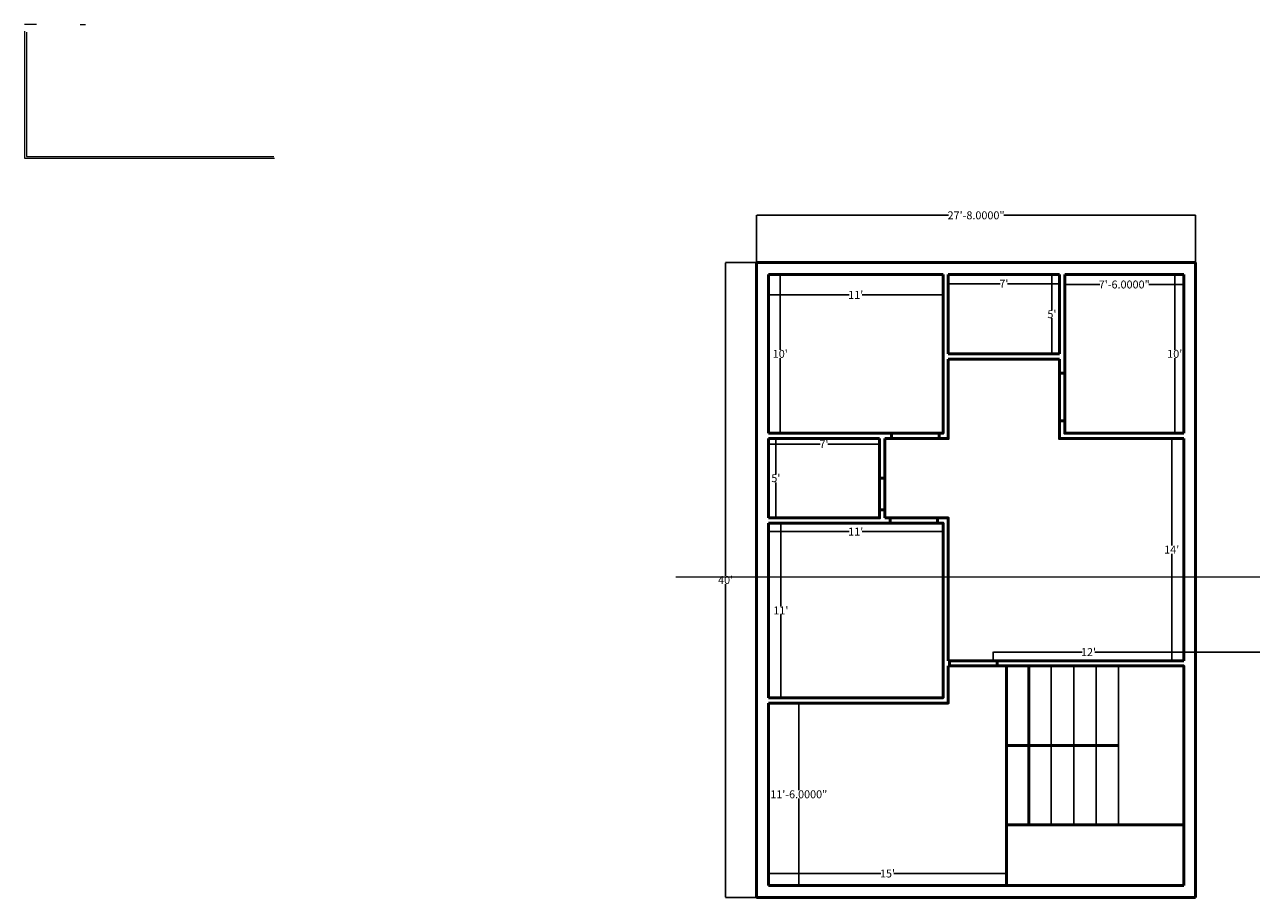
# Model space of a CAD drawing. Units: feet. Extents: x 993 to 3080, y -271 to 22562.
# Tile 2 of 4: x 993 to 1920, y 557 to 1217. Entities that reach past the tile are written whole.
import ezdxf

# ---------------------------------------------------------------- set-up
doc = ezdxf.new("R2010")
doc.units = ezdxf.units.FT
for name, color, linetype, lineweight in [('A-ANNO-DIMS', 2, 'Continuous', 18), ('A-ANNO-NPLT', 9, 'Continuous', 13), ('A-ANNO-SYMB', 4, 'Continuous', 18), ('A-FLOR-STRS', 3, 'Continuous', 25), ('A-WALL', 7, 'Continuous', 50)]:
    doc.layers.add(name, color=color, linetype=linetype, lineweight=lineweight)
doc.styles.get("Standard").update_dxf_attribs({"font": 'arial.ttf'})
doc.dimstyles.get("Standard").update_dxf_attribs({"dimtxt": 6, "dimasz": 0.18, "dimexe": 0.18, "dimexo": 0.0625, "dimgap": 0.09, "dimtad": 0, "dimtih": 1, "dimtoh": 1, "dimdec": 4, "dimzin": 0, "dimdsep": 46, "dimlunit": 3, "dimtxsty": 'Standard', "dimcen": 0.09, "dimadec": 0, "dimazin": 0, "dimtfac": 1, "dimtdec": 4, "dimtofl": 0, "dimtmove": 0, "dimatfit": 3, "dimfxl": 1, "dimtolj": 1, "dimtzin": 0, "dimarcsym": 0})

# ---------------------------------------------------------------- blocks, each defined once
blk = doc.blocks.new('*D1')
at = {"layer": 'A-ANNO-DIMS', "color": 0, "lineweight": -2, "transparency": 16777216}
for p, q in [((1545.92, 1037.12), (1545.92, 1072.98)), ((1546.1, 1072.8), (1690.98, 1072.8)), ((1877.74, 1072.8), (1732.85, 1072.8)), ((1877.92, 1037.12), (1877.92, 1072.98))]:
    blk.add_line(p, q, dxfattribs=at)
at = {"layer": 'A-ANNO-DIMS', "color": 0, "transparency": 16777216}
for points in [[(1546.1, 1072.83), (1546.1, 1072.77), (1545.92, 1072.8)], [(1877.74, 1072.83), (1877.74, 1072.77), (1877.92, 1072.8)]]:
    blk.add_solid(points, dxfattribs=at)
at = {"layer": 'Defpoints', "color": 0, "transparency": 16777216}
for p in [(1877.92, 1072.8), (1545.92, 1037.06), (1877.92, 1037.06)]:
    blk.add_point(p, dxfattribs=at)
at = {"layer": 'A-ANNO-DIMS', "color": 0, "transparency": 16777216, "insert": (1711.92, 1072.8), "char_height": 6, "attachment_point": 5}
blk.add_mtext('\\A1;27\'-8.0000"', dxfattribs=at)
blk = doc.blocks.new('*D2')
at = {"layer": 'A-ANNO-DIMS', "color": 0, "lineweight": -2, "transparency": 16777216}
for p, q in [((1545.85, 1037.06), (1522.38, 1037.06)), ((1522.56, 1036.88), (1522.56, 800.21)), ((1522.56, 557.24), (1522.56, 793.91)), ((1545.85, 557.06), (1522.38, 557.06))]:
    blk.add_line(p, q, dxfattribs=at)
at = {"layer": 'A-ANNO-DIMS', "color": 0, "transparency": 16777216}
for points in [[(1522.53, 1036.88), (1522.59, 1036.88), (1522.56, 1037.06)], [(1522.53, 557.24), (1522.59, 557.24), (1522.56, 557.06)]]:
    blk.add_solid(points, dxfattribs=at)
at = {"layer": 'Defpoints', "color": 0, "transparency": 16777216}
for p in [(1545.92, 1037.06), (1522.56, 557.06), (1545.92, 557.06)]:
    blk.add_point(p, dxfattribs=at)
at = {"layer": 'A-ANNO-DIMS', "color": 0, "transparency": 16777216, "insert": (1522.56, 797.06), "char_height": 6, "attachment_point": 5}
blk.add_mtext("\\A1;40'", dxfattribs=at)
blk = doc.blocks.new('*D3')
at = {"layer": 'A-ANNO-DIMS', "color": 0, "lineweight": -2, "transparency": 16777216}
for p, q in [((1554.92, 1028), (1554.92, 1012.47)), ((1686.92, 1028), (1686.92, 1012.47)), ((1555.1, 1012.65), (1616.02, 1012.65)), ((1686.74, 1012.65), (1625.81, 1012.65))]:
    blk.add_line(p, q, dxfattribs=at)
at = {"layer": 'A-ANNO-DIMS', "color": 0, "transparency": 16777216}
for points in [[(1555.1, 1012.68), (1555.1, 1012.62), (1554.92, 1012.65)], [(1686.74, 1012.68), (1686.74, 1012.62), (1686.92, 1012.65)]]:
    blk.add_solid(points, dxfattribs=at)
at = {"layer": 'Defpoints', "color": 0, "transparency": 16777216}
for p in [(1554.92, 1028.06), (1686.92, 1028.06), (1686.92, 1012.65)]:
    blk.add_point(p, dxfattribs=at)
at = {"layer": 'A-ANNO-DIMS', "color": 0, "transparency": 16777216, "insert": (1620.92, 1012.65), "char_height": 6, "attachment_point": 5}
blk.add_mtext("\\A1;11'", dxfattribs=at)
blk = doc.blocks.new('*D4')
at = {"layer": 'A-ANNO-DIMS', "color": 0, "lineweight": -2, "transparency": 16777216}
for p, q in [((1554.98, 1028.06), (1564.08, 1028.06)), ((1563.9, 1027.88), (1563.9, 971.21)), ((1563.9, 908.24), (1563.9, 964.91)), ((1554.98, 908.06), (1564.08, 908.06))]:
    blk.add_line(p, q, dxfattribs=at)
at = {"layer": 'A-ANNO-DIMS', "color": 0, "transparency": 16777216}
for points in [[(1563.87, 1027.88), (1563.93, 1027.88), (1563.9, 1028.06)], [(1563.87, 908.24), (1563.93, 908.24), (1563.9, 908.06)]]:
    blk.add_solid(points, dxfattribs=at)
at = {"layer": 'Defpoints', "color": 0, "transparency": 16777216}
for p in [(1554.92, 1028.06), (1554.92, 908.06), (1563.9, 908.06)]:
    blk.add_point(p, dxfattribs=at)
at = {"layer": 'A-ANNO-DIMS', "color": 0, "transparency": 16777216, "insert": (1563.9, 968.06), "char_height": 6, "attachment_point": 5}
blk.add_mtext("\\A1;10'", dxfattribs=at)
blk = doc.blocks.new('*D5')
at = {"layer": 'A-ANNO-DIMS', "color": 0, "lineweight": -2, "transparency": 16777216}
for p, q in [((1690.92, 1028), (1690.92, 1020.88)), ((1691.1, 1021.06), (1730.09, 1021.06)), ((1774.74, 1021.06), (1735.74, 1021.06)), ((1774.92, 1028), (1774.92, 1020.88))]:
    blk.add_line(p, q, dxfattribs=at)
at = {"layer": 'A-ANNO-DIMS', "color": 0, "transparency": 16777216}
for points in [[(1691.1, 1021.09), (1691.1, 1021.03), (1690.92, 1021.06)], [(1774.74, 1021.09), (1774.74, 1021.03), (1774.92, 1021.06)]]:
    blk.add_solid(points, dxfattribs=at)
at = {"layer": 'Defpoints', "color": 0, "transparency": 16777216}
for p in [(1690.92, 1028.06), (1774.92, 1028.06), (1774.92, 1021.06)]:
    blk.add_point(p, dxfattribs=at)
at = {"layer": 'A-ANNO-DIMS', "color": 0, "transparency": 16777216, "insert": (1732.92, 1021.06), "char_height": 6, "attachment_point": 5}
blk.add_mtext("\\A1;7'", dxfattribs=at)
blk = doc.blocks.new('*D6')
at = {"layer": 'A-ANNO-DIMS', "color": 0, "lineweight": -2, "transparency": 16777216}
for p, q in [((1774.85, 1028.06), (1769.08, 1028.06)), ((1769.26, 1027.88), (1769.26, 1001.2)), ((1769.26, 968.24), (1769.26, 994.92)), ((1774.85, 968.06), (1769.08, 968.06))]:
    blk.add_line(p, q, dxfattribs=at)
at = {"layer": 'A-ANNO-DIMS', "color": 0, "transparency": 16777216}
for points in [[(1769.23, 1027.88), (1769.29, 1027.88), (1769.26, 1028.06)], [(1769.23, 968.24), (1769.29, 968.24), (1769.26, 968.06)]]:
    blk.add_solid(points, dxfattribs=at)
at = {"layer": 'Defpoints', "color": 0, "transparency": 16777216}
for p in [(1769.26, 1028.06), (1774.92, 1028.06), (1774.92, 968.06)]:
    blk.add_point(p, dxfattribs=at)
at = {"layer": 'A-ANNO-DIMS', "color": 0, "transparency": 16777216, "insert": (1769.26, 998.06), "char_height": 6, "attachment_point": 5}
blk.add_mtext("\\A1;5'", dxfattribs=at)
blk = doc.blocks.new('*D7')
at = {"layer": 'A-ANNO-DIMS', "color": 0, "lineweight": -2, "transparency": 16777216}
for p, q in [((1778.92, 1028), (1778.92, 1020.32)), ((1779.1, 1020.5), (1805.39, 1020.5)), ((1868.74, 1020.5), (1842.44, 1020.5)), ((1868.92, 1028), (1868.92, 1020.32))]:
    blk.add_line(p, q, dxfattribs=at)
at = {"layer": 'A-ANNO-DIMS', "color": 0, "transparency": 16777216}
for points in [[(1779.1, 1020.53), (1779.1, 1020.47), (1778.92, 1020.5)], [(1868.74, 1020.53), (1868.74, 1020.47), (1868.92, 1020.5)]]:
    blk.add_solid(points, dxfattribs=at)
at = {"layer": 'Defpoints', "color": 0, "transparency": 16777216}
for p in [(1778.92, 1028.06), (1778.92, 1020.5), (1868.92, 1028.06)]:
    blk.add_point(p, dxfattribs=at)
at = {"layer": 'A-ANNO-DIMS', "color": 0, "transparency": 16777216, "insert": (1823.92, 1020.5), "char_height": 6, "attachment_point": 5}
blk.add_mtext('\\A1;7\'-6.0000"', dxfattribs=at)
blk = doc.blocks.new('*D8')
at = {"layer": 'A-ANNO-DIMS', "color": 0, "lineweight": -2, "transparency": 16777216}
for p, q in [((1868.85, 1028.06), (1861.9, 1028.06)), ((1862.08, 1027.88), (1862.08, 971.21)), ((1862.08, 908.24), (1862.08, 964.91)), ((1868.85, 908.06), (1861.9, 908.06))]:
    blk.add_line(p, q, dxfattribs=at)
at = {"layer": 'A-ANNO-DIMS', "color": 0, "transparency": 16777216}
for points in [[(1862.05, 1027.88), (1862.11, 1027.88), (1862.08, 1028.06)], [(1862.05, 908.24), (1862.11, 908.24), (1862.08, 908.06)]]:
    blk.add_solid(points, dxfattribs=at)
at = {"layer": 'Defpoints', "color": 0, "transparency": 16777216}
for p in [(1868.92, 1028.06), (1862.08, 908.06), (1868.92, 908.06)]:
    blk.add_point(p, dxfattribs=at)
at = {"layer": 'A-ANNO-DIMS', "color": 0, "transparency": 16777216, "insert": (1862.08, 968.06), "char_height": 6, "attachment_point": 5}
blk.add_mtext("\\A1;10'", dxfattribs=at)
blk = doc.blocks.new('*D9')
at = {"layer": 'A-ANNO-DIMS', "color": 0, "lineweight": -2, "transparency": 16777216}
for p, q in [((1554.92, 904), (1554.92, 899.62)), ((1555.1, 899.8), (1594.09, 899.8)), ((1638.74, 899.8), (1599.74, 899.8)), ((1638.92, 904), (1638.92, 899.62))]:
    blk.add_line(p, q, dxfattribs=at)
at = {"layer": 'A-ANNO-DIMS', "color": 0, "transparency": 16777216}
for points in [[(1555.1, 899.83), (1555.1, 899.77), (1554.92, 899.8)], [(1638.74, 899.83), (1638.74, 899.77), (1638.92, 899.8)]]:
    blk.add_solid(points, dxfattribs=at)
at = {"layer": 'Defpoints', "color": 0, "transparency": 16777216}
for p in [(1554.92, 904.06), (1554.92, 899.8), (1638.92, 904.06)]:
    blk.add_point(p, dxfattribs=at)
at = {"layer": 'A-ANNO-DIMS', "color": 0, "transparency": 16777216, "insert": (1596.92, 899.8), "char_height": 6, "attachment_point": 5}
blk.add_mtext("\\A1;7'", dxfattribs=at)
blk = doc.blocks.new('*D10')
at = {"layer": 'A-ANNO-DIMS', "color": 0, "lineweight": -2, "transparency": 16777216}
for p, q in [((1554.98, 904.06), (1560.73, 904.06)), ((1560.55, 903.88), (1560.55, 877.2)), ((1560.55, 844.24), (1560.55, 870.92)), ((1554.98, 844.06), (1560.73, 844.06))]:
    blk.add_line(p, q, dxfattribs=at)
at = {"layer": 'A-ANNO-DIMS', "color": 0, "transparency": 16777216}
for points in [[(1560.52, 903.88), (1560.58, 903.88), (1560.55, 904.06)], [(1560.52, 844.24), (1560.58, 844.24), (1560.55, 844.06)]]:
    blk.add_solid(points, dxfattribs=at)
at = {"layer": 'Defpoints', "color": 0, "transparency": 16777216}
for p in [(1554.92, 904.06), (1554.92, 844.06), (1560.55, 844.06)]:
    blk.add_point(p, dxfattribs=at)
at = {"layer": 'A-ANNO-DIMS', "color": 0, "transparency": 16777216, "insert": (1560.55, 874.06), "char_height": 6, "attachment_point": 5}
blk.add_mtext("\\A1;5'", dxfattribs=at)
blk = doc.blocks.new('*D11')
at = {"layer": 'A-ANNO-DIMS', "color": 0, "lineweight": -2, "transparency": 16777216}
for p, q in [((1554.98, 840.06), (1564.54, 840.06)), ((1564.36, 839.88), (1564.36, 777.16)), ((1564.36, 708.24), (1564.36, 770.96)), ((1554.98, 708.06), (1564.54, 708.06))]:
    blk.add_line(p, q, dxfattribs=at)
at = {"layer": 'A-ANNO-DIMS', "color": 0, "transparency": 16777216}
for points in [[(1564.33, 839.88), (1564.39, 839.88), (1564.36, 840.06)], [(1564.33, 708.24), (1564.39, 708.24), (1564.36, 708.06)]]:
    blk.add_solid(points, dxfattribs=at)
at = {"layer": 'Defpoints', "color": 0, "transparency": 16777216}
for p in [(1554.92, 840.06), (1554.92, 708.06), (1564.36, 708.06)]:
    blk.add_point(p, dxfattribs=at)
at = {"layer": 'A-ANNO-DIMS', "color": 0, "transparency": 16777216, "insert": (1564.36, 774.06), "char_height": 6, "attachment_point": 5}
blk.add_mtext("\\A1;11'", dxfattribs=at)
blk = doc.blocks.new('*D12')
at = {"layer": 'A-ANNO-DIMS', "color": 0, "lineweight": -2, "transparency": 16777216}
for p, q in [((1554.92, 840), (1554.92, 833.46)), ((1686.92, 840), (1686.92, 833.46)), ((1555.1, 833.64), (1616.02, 833.64)), ((1686.74, 833.64), (1625.81, 833.64))]:
    blk.add_line(p, q, dxfattribs=at)
at = {"layer": 'A-ANNO-DIMS', "color": 0, "transparency": 16777216}
for points in [[(1555.1, 833.67), (1555.1, 833.61), (1554.92, 833.64)], [(1686.74, 833.67), (1686.74, 833.61), (1686.92, 833.64)]]:
    blk.add_solid(points, dxfattribs=at)
at = {"layer": 'Defpoints', "color": 0, "transparency": 16777216}
for p in [(1554.92, 840.06), (1686.92, 840.06), (1686.92, 833.64)]:
    blk.add_point(p, dxfattribs=at)
at = {"layer": 'A-ANNO-DIMS', "color": 0, "transparency": 16777216, "insert": (1620.92, 833.64), "char_height": 6, "attachment_point": 5}
blk.add_mtext("\\A1;11'", dxfattribs=at)
blk = doc.blocks.new('*D13')
at = {"layer": 'A-ANNO-DIMS', "color": 0, "lineweight": -2, "transparency": 16777216}
for p, q in [((1868.85, 904.06), (1859.63, 904.06)), ((1859.81, 903.88), (1859.81, 823.16)), ((1859.81, 736.24), (1859.81, 816.96)), ((1868.85, 736.06), (1859.63, 736.06))]:
    blk.add_line(p, q, dxfattribs=at)
at = {"layer": 'A-ANNO-DIMS', "color": 0, "transparency": 16777216}
for points in [[(1859.78, 903.88), (1859.84, 903.88), (1859.81, 904.06)], [(1859.78, 736.24), (1859.84, 736.24), (1859.81, 736.06)]]:
    blk.add_solid(points, dxfattribs=at)
at = {"layer": 'Defpoints', "color": 0, "transparency": 16777216}
for p in [(1868.92, 904.06), (1859.81, 736.06), (1868.92, 736.06)]:
    blk.add_point(p, dxfattribs=at)
at = {"layer": 'A-ANNO-DIMS', "color": 0, "transparency": 16777216, "insert": (1859.81, 820.06), "char_height": 6, "attachment_point": 5}
blk.add_mtext("\\A1;14'", dxfattribs=at)
blk = doc.blocks.new('*D14')
at = {"layer": 'A-ANNO-DIMS', "color": 0, "lineweight": -2, "transparency": 16777216}
for p, q in [((1724.92, 736.12), (1724.92, 742.78)), ((1725.1, 742.6), (1792.02, 742.6)), ((1868.74, 742.6), (1801.81, 742.6)), ((1868.92, 736.12), (1868.92, 742.78))]:
    blk.add_line(p, q, dxfattribs=at)
at = {"layer": 'A-ANNO-DIMS', "color": 0, "transparency": 16777216}
for points in [[(1725.1, 742.63), (1725.1, 742.57), (1724.92, 742.6)], [(1868.74, 742.63), (1868.74, 742.57), (1868.92, 742.6)]]:
    blk.add_solid(points, dxfattribs=at)
at = {"layer": 'Defpoints', "color": 0, "transparency": 16777216}
for p in [(1724.92, 742.6), (1724.92, 736.06), (1868.92, 736.06)]:
    blk.add_point(p, dxfattribs=at)
at = {"layer": 'A-ANNO-DIMS', "color": 0, "transparency": 16777216, "insert": (1796.92, 742.6), "char_height": 6, "attachment_point": 5}
blk.add_mtext("\\A1;12'", dxfattribs=at)
blk = doc.blocks.new('*D15')
at = {"layer": 'A-ANNO-DIMS', "color": 0, "lineweight": -2, "transparency": 16777216}
for p, q in [((1554.98, 704.06), (1578.06, 704.06)), ((1577.88, 703.88), (1577.88, 638.21)), ((1577.88, 566.24), (1577.88, 631.91)), ((1554.98, 566.06), (1578.06, 566.06))]:
    blk.add_line(p, q, dxfattribs=at)
at = {"layer": 'A-ANNO-DIMS', "color": 0, "transparency": 16777216}
for points in [[(1577.85, 703.88), (1577.91, 703.88), (1577.88, 704.06)], [(1577.85, 566.24), (1577.91, 566.24), (1577.88, 566.06)]]:
    blk.add_solid(points, dxfattribs=at)
at = {"layer": 'Defpoints', "color": 0, "transparency": 16777216}
for p in [(1554.92, 704.06), (1554.92, 566.06), (1577.88, 566.06)]:
    blk.add_point(p, dxfattribs=at)
at = {"layer": 'A-ANNO-DIMS', "color": 0, "transparency": 16777216, "insert": (1577.88, 635.06), "char_height": 6, "attachment_point": 5}
blk.add_mtext('\\A1;11\'-6.0000"', dxfattribs=at)
blk = doc.blocks.new('*D16')
at = {"layer": 'A-ANNO-DIMS', "color": 0, "lineweight": -2, "transparency": 16777216}
for p, q in [((1554.92, 566.12), (1554.92, 575.34)), ((1555.1, 575.16), (1640.02, 575.16)), ((1734.74, 575.16), (1649.81, 575.16)), ((1734.92, 566.12), (1734.92, 575.34))]:
    blk.add_line(p, q, dxfattribs=at)
at = {"layer": 'A-ANNO-DIMS', "color": 0, "transparency": 16777216}
for points in [[(1555.1, 575.19), (1555.1, 575.13), (1554.92, 575.16)], [(1734.74, 575.19), (1734.74, 575.13), (1734.92, 575.16)]]:
    blk.add_solid(points, dxfattribs=at)
at = {"layer": 'Defpoints', "color": 0, "transparency": 16777216}
for p in [(1734.92, 575.16), (1554.92, 566.06), (1734.92, 566.06)]:
    blk.add_point(p, dxfattribs=at)
at = {"layer": 'A-ANNO-DIMS', "color": 0, "transparency": 16777216, "insert": (1644.92, 575.16), "char_height": 6, "attachment_point": 5}
blk.add_mtext("\\A1;15'", dxfattribs=at)
blk = doc.blocks.new('*D19')
at = {"layer": 'A-ANNO-DIMS', "color": 0, "lineweight": -2, "transparency": 16777216}
for p, q in [((1554.92, 1028), (1554.92, 1012.47)), ((1686.92, 1028), (1686.92, 1012.47)), ((1555.1, 1012.65), (1616.02, 1012.65)), ((1686.74, 1012.65), (1625.81, 1012.65))]:
    blk.add_line(p, q, dxfattribs=at)
at = {"layer": 'A-ANNO-DIMS', "color": 0, "transparency": 16777216}
for points in [[(1555.1, 1012.68), (1555.1, 1012.62), (1554.92, 1012.65)], [(1686.74, 1012.68), (1686.74, 1012.62), (1686.92, 1012.65)]]:
    blk.add_solid(points, dxfattribs=at)
at = {"layer": 'Defpoints', "color": 0, "transparency": 16777216}
for p in [(1554.92, 1028.06), (1686.92, 1028.06), (1686.92, 1012.65)]:
    blk.add_point(p, dxfattribs=at)
at = {"layer": 'A-ANNO-DIMS', "color": 0, "transparency": 16777216, "insert": (1620.92, 1012.65), "char_height": 6, "attachment_point": 5}
blk.add_mtext("\\A1;11'", dxfattribs=at)
blk = doc.blocks.new('*D20')
at = {"layer": 'A-ANNO-DIMS', "color": 0, "lineweight": -2, "transparency": 16777216}
for p, q in [((1554.98, 1028.06), (1564.08, 1028.06)), ((1563.9, 1027.88), (1563.9, 971.21)), ((1563.9, 908.24), (1563.9, 964.91)), ((1554.98, 908.06), (1564.08, 908.06))]:
    blk.add_line(p, q, dxfattribs=at)
at = {"layer": 'A-ANNO-DIMS', "color": 0, "transparency": 16777216}
for points in [[(1563.87, 1027.88), (1563.93, 1027.88), (1563.9, 1028.06)], [(1563.87, 908.24), (1563.93, 908.24), (1563.9, 908.06)]]:
    blk.add_solid(points, dxfattribs=at)
at = {"layer": 'Defpoints', "color": 0, "transparency": 16777216}
for p in [(1554.92, 1028.06), (1554.92, 908.06), (1563.9, 908.06)]:
    blk.add_point(p, dxfattribs=at)
at = {"layer": 'A-ANNO-DIMS', "color": 0, "transparency": 16777216, "insert": (1563.9, 968.06), "char_height": 6, "attachment_point": 5}
blk.add_mtext("\\A1;10'", dxfattribs=at)
blk = doc.blocks.new('*D21')
at = {"layer": 'A-ANNO-DIMS', "color": 0, "lineweight": -2, "transparency": 16777216}
for p, q in [((1690.92, 1028), (1690.92, 1020.88)), ((1691.1, 1021.06), (1730.09, 1021.06)), ((1774.74, 1021.06), (1735.74, 1021.06)), ((1774.92, 1028), (1774.92, 1020.88))]:
    blk.add_line(p, q, dxfattribs=at)
at = {"layer": 'A-ANNO-DIMS', "color": 0, "transparency": 16777216}
for points in [[(1691.1, 1021.09), (1691.1, 1021.03), (1690.92, 1021.06)], [(1774.74, 1021.09), (1774.74, 1021.03), (1774.92, 1021.06)]]:
    blk.add_solid(points, dxfattribs=at)
at = {"layer": 'Defpoints', "color": 0, "transparency": 16777216}
for p in [(1690.92, 1028.06), (1774.92, 1028.06), (1774.92, 1021.06)]:
    blk.add_point(p, dxfattribs=at)
at = {"layer": 'A-ANNO-DIMS', "color": 0, "transparency": 16777216, "insert": (1732.92, 1021.06), "char_height": 6, "attachment_point": 5}
blk.add_mtext("\\A1;7'", dxfattribs=at)
blk = doc.blocks.new('*D22')
at = {"layer": 'A-ANNO-DIMS', "color": 0, "lineweight": -2, "transparency": 16777216}
for p, q in [((1774.85, 1028.06), (1769.08, 1028.06)), ((1769.26, 1027.88), (1769.26, 1001.2)), ((1769.26, 968.24), (1769.26, 994.92)), ((1774.85, 968.06), (1769.08, 968.06))]:
    blk.add_line(p, q, dxfattribs=at)
at = {"layer": 'A-ANNO-DIMS', "color": 0, "transparency": 16777216}
for points in [[(1769.23, 1027.88), (1769.29, 1027.88), (1769.26, 1028.06)], [(1769.23, 968.24), (1769.29, 968.24), (1769.26, 968.06)]]:
    blk.add_solid(points, dxfattribs=at)
at = {"layer": 'Defpoints', "color": 0, "transparency": 16777216}
for p in [(1769.26, 1028.06), (1774.92, 1028.06), (1774.92, 968.06)]:
    blk.add_point(p, dxfattribs=at)
at = {"layer": 'A-ANNO-DIMS', "color": 0, "transparency": 16777216, "insert": (1769.26, 998.06), "char_height": 6, "attachment_point": 5}
blk.add_mtext("\\A1;5'", dxfattribs=at)
blk = doc.blocks.new('*D23')
at = {"layer": 'A-ANNO-DIMS', "color": 0, "lineweight": -2, "transparency": 16777216}
for p, q in [((1778.92, 1028), (1778.92, 1020.32)), ((1779.1, 1020.5), (1805.39, 1020.5)), ((1868.74, 1020.5), (1842.44, 1020.5)), ((1868.92, 1028), (1868.92, 1020.32))]:
    blk.add_line(p, q, dxfattribs=at)
at = {"layer": 'A-ANNO-DIMS', "color": 0, "transparency": 16777216}
for points in [[(1779.1, 1020.53), (1779.1, 1020.47), (1778.92, 1020.5)], [(1868.74, 1020.53), (1868.74, 1020.47), (1868.92, 1020.5)]]:
    blk.add_solid(points, dxfattribs=at)
at = {"layer": 'Defpoints', "color": 0, "transparency": 16777216}
for p in [(1778.92, 1028.06), (1778.92, 1020.5), (1868.92, 1028.06)]:
    blk.add_point(p, dxfattribs=at)
at = {"layer": 'A-ANNO-DIMS', "color": 0, "transparency": 16777216, "insert": (1823.92, 1020.5), "char_height": 6, "attachment_point": 5}
blk.add_mtext('\\A1;7\'-6.0000"', dxfattribs=at)
blk = doc.blocks.new('*D24')
at = {"layer": 'A-ANNO-DIMS', "color": 0, "lineweight": -2, "transparency": 16777216}
for p, q in [((1868.85, 1028.06), (1861.9, 1028.06)), ((1862.08, 1027.88), (1862.08, 971.21)), ((1862.08, 908.24), (1862.08, 964.91)), ((1868.85, 908.06), (1861.9, 908.06))]:
    blk.add_line(p, q, dxfattribs=at)
at = {"layer": 'A-ANNO-DIMS', "color": 0, "transparency": 16777216}
for points in [[(1862.05, 1027.88), (1862.11, 1027.88), (1862.08, 1028.06)], [(1862.05, 908.24), (1862.11, 908.24), (1862.08, 908.06)]]:
    blk.add_solid(points, dxfattribs=at)
at = {"layer": 'Defpoints', "color": 0, "transparency": 16777216}
for p in [(1868.92, 1028.06), (1862.08, 908.06), (1868.92, 908.06)]:
    blk.add_point(p, dxfattribs=at)
at = {"layer": 'A-ANNO-DIMS', "color": 0, "transparency": 16777216, "insert": (1862.08, 968.06), "char_height": 6, "attachment_point": 5}
blk.add_mtext("\\A1;10'", dxfattribs=at)
blk = doc.blocks.new('*D25')
at = {"layer": 'A-ANNO-DIMS', "color": 0, "lineweight": -2, "transparency": 16777216}
for p, q in [((1554.92, 904), (1554.92, 899.62)), ((1555.1, 899.8), (1594.09, 899.8)), ((1638.74, 899.8), (1599.74, 899.8)), ((1638.92, 904), (1638.92, 899.62))]:
    blk.add_line(p, q, dxfattribs=at)
at = {"layer": 'A-ANNO-DIMS', "color": 0, "transparency": 16777216}
for points in [[(1555.1, 899.83), (1555.1, 899.77), (1554.92, 899.8)], [(1638.74, 899.83), (1638.74, 899.77), (1638.92, 899.8)]]:
    blk.add_solid(points, dxfattribs=at)
at = {"layer": 'Defpoints', "color": 0, "transparency": 16777216}
for p in [(1554.92, 904.06), (1554.92, 899.8), (1638.92, 904.06)]:
    blk.add_point(p, dxfattribs=at)
at = {"layer": 'A-ANNO-DIMS', "color": 0, "transparency": 16777216, "insert": (1596.92, 899.8), "char_height": 6, "attachment_point": 5}
blk.add_mtext("\\A1;7'", dxfattribs=at)
blk = doc.blocks.new('*D26')
at = {"layer": 'A-ANNO-DIMS', "color": 0, "lineweight": -2, "transparency": 16777216}
for p, q in [((1554.98, 904.06), (1560.73, 904.06)), ((1560.55, 903.88), (1560.55, 877.2)), ((1560.55, 844.24), (1560.55, 870.92)), ((1554.98, 844.06), (1560.73, 844.06))]:
    blk.add_line(p, q, dxfattribs=at)
at = {"layer": 'A-ANNO-DIMS', "color": 0, "transparency": 16777216}
for points in [[(1560.52, 903.88), (1560.58, 903.88), (1560.55, 904.06)], [(1560.52, 844.24), (1560.58, 844.24), (1560.55, 844.06)]]:
    blk.add_solid(points, dxfattribs=at)
at = {"layer": 'Defpoints', "color": 0, "transparency": 16777216}
for p in [(1554.92, 904.06), (1554.92, 844.06), (1560.55, 844.06)]:
    blk.add_point(p, dxfattribs=at)
at = {"layer": 'A-ANNO-DIMS', "color": 0, "transparency": 16777216, "insert": (1560.55, 874.06), "char_height": 6, "attachment_point": 5}
blk.add_mtext("\\A1;5'", dxfattribs=at)
blk = doc.blocks.new('*D27')
at = {"layer": 'A-ANNO-DIMS', "color": 0, "lineweight": -2, "transparency": 16777216}
for p, q in [((1554.98, 840.06), (1564.54, 840.06)), ((1564.36, 839.88), (1564.36, 777.16)), ((1564.36, 708.24), (1564.36, 770.96)), ((1554.98, 708.06), (1564.54, 708.06))]:
    blk.add_line(p, q, dxfattribs=at)
at = {"layer": 'A-ANNO-DIMS', "color": 0, "transparency": 16777216}
for points in [[(1564.33, 839.88), (1564.39, 839.88), (1564.36, 840.06)], [(1564.33, 708.24), (1564.39, 708.24), (1564.36, 708.06)]]:
    blk.add_solid(points, dxfattribs=at)
at = {"layer": 'Defpoints', "color": 0, "transparency": 16777216}
for p in [(1554.92, 840.06), (1554.92, 708.06), (1564.36, 708.06)]:
    blk.add_point(p, dxfattribs=at)
at = {"layer": 'A-ANNO-DIMS', "color": 0, "transparency": 16777216, "insert": (1564.36, 774.06), "char_height": 6, "attachment_point": 5}
blk.add_mtext("\\A1;11'", dxfattribs=at)
blk = doc.blocks.new('*D28')
at = {"layer": 'A-ANNO-DIMS', "color": 0, "lineweight": -2, "transparency": 16777216}
for p, q in [((1554.92, 840), (1554.92, 833.46)), ((1686.92, 840), (1686.92, 833.46)), ((1555.1, 833.64), (1616.02, 833.64)), ((1686.74, 833.64), (1625.81, 833.64))]:
    blk.add_line(p, q, dxfattribs=at)
at = {"layer": 'A-ANNO-DIMS', "color": 0, "transparency": 16777216}
for points in [[(1555.1, 833.67), (1555.1, 833.61), (1554.92, 833.64)], [(1686.74, 833.67), (1686.74, 833.61), (1686.92, 833.64)]]:
    blk.add_solid(points, dxfattribs=at)
at = {"layer": 'Defpoints', "color": 0, "transparency": 16777216}
for p in [(1554.92, 840.06), (1686.92, 840.06), (1686.92, 833.64)]:
    blk.add_point(p, dxfattribs=at)
at = {"layer": 'A-ANNO-DIMS', "color": 0, "transparency": 16777216, "insert": (1620.92, 833.64), "char_height": 6, "attachment_point": 5}
blk.add_mtext("\\A1;11'", dxfattribs=at)
blk = doc.blocks.new('*D29')
at = {"layer": 'A-ANNO-DIMS', "color": 0, "lineweight": -2, "transparency": 16777216}
for p, q in [((1868.85, 904.06), (1859.63, 904.06)), ((1859.81, 903.88), (1859.81, 823.16)), ((1859.81, 736.24), (1859.81, 816.96)), ((1868.85, 736.06), (1859.63, 736.06))]:
    blk.add_line(p, q, dxfattribs=at)
at = {"layer": 'A-ANNO-DIMS', "color": 0, "transparency": 16777216}
for points in [[(1859.78, 903.88), (1859.84, 903.88), (1859.81, 904.06)], [(1859.78, 736.24), (1859.84, 736.24), (1859.81, 736.06)]]:
    blk.add_solid(points, dxfattribs=at)
at = {"layer": 'Defpoints', "color": 0, "transparency": 16777216}
for p in [(1868.92, 904.06), (1859.81, 736.06), (1868.92, 736.06)]:
    blk.add_point(p, dxfattribs=at)
at = {"layer": 'A-ANNO-DIMS', "color": 0, "transparency": 16777216, "insert": (1859.81, 820.06), "char_height": 6, "attachment_point": 5}
blk.add_mtext("\\A1;14'", dxfattribs=at)
blk = doc.blocks.new('*D30')
at = {"layer": 'A-ANNO-DIMS', "color": 0, "lineweight": -2, "transparency": 16777216}
for p, q in [((1868.92, 736.12), (1868.92, 742.78)), ((1869.1, 742.6), (1999, 742.6)), ((2170.78, 742.6), (2040.87, 742.6)), ((2170.96, 736.12), (2170.96, 742.78))]:
    blk.add_line(p, q, dxfattribs=at)
at = {"layer": 'A-ANNO-DIMS', "color": 0, "transparency": 16777216}
for points in [[(1869.1, 742.63), (1869.1, 742.57), (1868.92, 742.6)], [(2170.78, 742.63), (2170.78, 742.57), (2170.96, 742.6)]]:
    blk.add_solid(points, dxfattribs=at)
at = {"layer": 'Defpoints', "color": 0, "transparency": 16777216}
for p in [(2170.96, 742.6), (1868.92, 736.06), (2170.96, 736.06)]:
    blk.add_point(p, dxfattribs=at)
at = {"layer": 'A-ANNO-DIMS', "color": 0, "transparency": 16777216, "insert": (2019.94, 742.6), "char_height": 6, "attachment_point": 5}
blk.add_mtext('\\A1;25\'-2.0427"', dxfattribs=at)
blk = doc.blocks.new('*D31')
at = {"layer": 'A-ANNO-DIMS', "color": 0, "lineweight": -2, "transparency": 16777216}
for p, q in [((1554.98, 704.06), (1578.06, 704.06)), ((1577.88, 703.88), (1577.88, 638.21)), ((1577.88, 566.24), (1577.88, 631.91)), ((1554.98, 566.06), (1578.06, 566.06))]:
    blk.add_line(p, q, dxfattribs=at)
at = {"layer": 'A-ANNO-DIMS', "color": 0, "transparency": 16777216}
for points in [[(1577.85, 703.88), (1577.91, 703.88), (1577.88, 704.06)], [(1577.85, 566.24), (1577.91, 566.24), (1577.88, 566.06)]]:
    blk.add_solid(points, dxfattribs=at)
at = {"layer": 'Defpoints', "color": 0, "transparency": 16777216}
for p in [(1554.92, 704.06), (1554.92, 566.06), (1577.88, 566.06)]:
    blk.add_point(p, dxfattribs=at)
at = {"layer": 'A-ANNO-DIMS', "color": 0, "transparency": 16777216, "insert": (1577.88, 635.06), "char_height": 6, "attachment_point": 5}
blk.add_mtext('\\A1;11\'-6.0000"', dxfattribs=at)
blk = doc.blocks.new('*D32')
at = {"layer": 'A-ANNO-DIMS', "color": 0, "lineweight": -2, "transparency": 16777216}
for p, q in [((1554.92, 566.12), (1554.92, 575.34)), ((1555.1, 575.16), (1640.02, 575.16)), ((1734.74, 575.16), (1649.81, 575.16)), ((1734.92, 566.12), (1734.92, 575.34))]:
    blk.add_line(p, q, dxfattribs=at)
at = {"layer": 'A-ANNO-DIMS', "color": 0, "transparency": 16777216}
for points in [[(1555.1, 575.19), (1555.1, 575.13), (1554.92, 575.16)], [(1734.74, 575.19), (1734.74, 575.13), (1734.92, 575.16)]]:
    blk.add_solid(points, dxfattribs=at)
at = {"layer": 'Defpoints', "color": 0, "transparency": 16777216}
for p in [(1734.92, 575.16), (1554.92, 566.06), (1734.92, 566.06)]:
    blk.add_point(p, dxfattribs=at)
at = {"layer": 'A-ANNO-DIMS', "color": 0, "transparency": 16777216, "insert": (1644.92, 575.16), "char_height": 6, "attachment_point": 5}
blk.add_mtext("\\A1;15'", dxfattribs=at)

msp = doc.modelspace()

# ---------------------------------------------------------------- linework, layer by layer
at = {"layer": 'A-ANNO-NPLT'}
for p, q in [((1001.57081, 1217.04014, 120), (992.57081, 1217.04014, 120)), ((1034.5813, 1217.04014, 120), (1038.5813, 1217.04014, 120))]:
    msp.add_line(p, q, dxfattribs=at)
for points, elevation in [([(992.57081, 1212.04014), (992.57081, 1116.04014), (1181.57081, 1116.04014)], 186), ([(992.57081, 1212.04014), (992.57081, 1116.04014), (1181.57081, 1116.04014)], 312), ([(994.12395, 1211.29263), (994.12395, 1117.29263), (1181.12395, 1117.29263)], 186), ([(994.12395, 1211.29263), (994.12395, 1117.29263), (1181.12395, 1117.29263)], 312)]:
    msp.add_lwpolyline(points, dxfattribs=dict(at, elevation=elevation))
at = {"layer": 'A-ANNO-SYMB'}
msp.add_line((1484.89473, 799.38224), (2862.87672, 799.38224), dxfattribs=at)
at = {"layer": 'A-FLOR-STRS'}
for p, q in [((1768.80081, 732.05993), (1768.80081, 612.05993)), ((1785.74369, 732.05993), (1785.74369, 612.05993)), ((1802.68657, 732.05993), (1802.68657, 612.05993)), ((1819.62945, 732.05993), (1819.62945, 612.05993))]:
    msp.add_line(p, q, dxfattribs=at)
at = {"layer": 'A-FLOR-STRS', "extrusion": (0, -1, 0)}
msp.add_line((1819.62945, 612.05993), (1819.62945, 732.05993), dxfattribs=at)
at = {"layer": 'A-WALL'}
for p, q in [((1868.91505, 908.05993), (1868.91505, 1028.05993)), ((1868.91505, 736.05993), (1868.91505, 904.05993)), ((1734.91505, 566.05993), (1734.91505, 732.05993)), ((1734.91505, 732.05993), (1734.91505, 612.05993)), ((1751.85793, 732.05993), (1751.85793, 612.05993)), ((1734.91505, 672.05993), (1819.62945, 672.05993)), ((1734.91505, 612.05993), (1868.91505, 612.05993))]:
    msp.add_line(p, q, dxfattribs=at)
at = {"layer": 'A-WALL', "extrusion": (0, -1, 0)}
for p, q in [((1819.62945, 732.05993), (1868.91505, 732.05993)), ((1868.91505, 732.05993), (1868.91505, 612.05993)), ((1868.91505, 612.05993), (1819.62945, 612.05993))]:
    msp.add_line(p, q, dxfattribs=at)
at = {"layer": 'A-WALL'}
for points in [[(1545.91505, 1037.05993), (1877.91505, 1037.05993)], [(1545.91505, 557.05993), (1545.91505, 1037.05993)], [(1877.91505, 1037.05993), (1877.91505, 557.05993)], [(1554.91505, 1028.05993), (1686.91505, 1028.05993)], [(1554.91505, 908.05993), (1554.91505, 1028.05993)], [(1686.91505, 1028.05993), (1686.91505, 908.05993), (1554.91505, 908.05993)], [(1690.91505, 1028.05993), (1774.91505, 1028.05993)], [(1690.91505, 1028.05993), (1690.91505, 968.05993)], [(1774.91505, 1028.05993), (1774.91505, 968.05993)], [(1778.91505, 1028.05993), (1868.91505, 1028.05993)], [(1778.91505, 1028.05993), (1778.91505, 908.05993), (1868.91505, 908.05993)], [(1868.91505, 1028.05993), (1868.91505, 908.05993)], [(1774.91505, 968.05993), (1690.91505, 968.05993)], [(1690.91505, 964.05993), (1690.91505, 904.05993), (1642.91505, 904.05993)], [(1774.91505, 964.05993), (1690.91505, 964.05993)], [(1774.91505, 964.05993), (1774.91505, 904.05993), (1868.91505, 904.05993)], [(1554.91505, 844.05993), (1554.91505, 904.05993)], [(1638.91505, 904.05993), (1554.91505, 904.05993)], [(1638.91505, 904.05993), (1638.91505, 844.05993), (1554.91505, 844.05993)], [(1642.91505, 904.05993), (1642.91505, 844.05993)], [(1868.91505, 904.05993), (1774.91505, 904.05993)], [(1868.91505, 908.05993), (1778.91505, 908.05993)], [(1868.91505, 904.05993), (1868.91505, 736.05993)], [(1690.91505, 736.05993), (1690.91505, 844.05993), (1642.91505, 844.05993)], [(1554.91505, 708.05993), (1554.91505, 840.05993)], [(1642.91505, 840.05993), (1554.91505, 840.05993)], [(1554.91505, 708.05993), (1686.91505, 708.05993), (1686.91505, 840.05993), (1642.91505, 840.05993)], [(1690.91505, 736.05993), (1868.91505, 736.05993)], [(1554.91505, 704.05993), (1690.91505, 704.05993), (1690.91505, 732.05993)], [(1690.91505, 732.05993), (1868.91505, 732.05993)], [(1868.91505, 732.05993), (1868.91505, 566.05993)], [(1554.91505, 566.05993), (1554.91505, 704.05993)], [(1868.91505, 566.05993), (1554.91505, 566.05993)], [(1877.91505, 557.05993), (1545.91505, 557.05993)]]:
    msp.add_lwpolyline(points, dxfattribs=at)
for points in [[(1774.91505, 953.34554), (1778.91505, 953.34554), (1778.91505, 917.34554), (1774.91505, 917.34554)], [(1684.01445, 908.05993), (1684.01445, 904.05993), (1648.01445, 904.05993), (1648.01445, 908.05993)], [(1643.00422, 874.05993), (1643.00422, 850.05993), (1639.00422, 850.05993), (1639.00422, 874.05993)], [(1682.86453, 844.05993), (1682.86453, 840.05993), (1646.86453, 840.05993), (1646.86453, 844.05993)], [(1727.79457, 736.05993), (1727.79457, 732.05993), (1691.79457, 732.05993), (1691.79457, 736.05993)]]:
    msp.add_lwpolyline(points, close=True, dxfattribs=at)
at = {"layer": 'A-WALL', "extrusion": (0, -1, 0), "elevation": -732.05993}
msp.add_lwpolyline([(1819.62945, 0), (1868.91505, 0), (1868.91505, 0), (1819.62945, 0)], close=True, dxfattribs=at)

# ---------------------------------------------------------------- dimensions: what is measured, and where the dimension line sits
at = {"layer": 'A-ANNO-DIMS'}
for base, p1, p2, picture, middle in [((1877.91505, 1072.79599), (1545.91505, 1037.05993), (1877.91505, 1037.05993), '*D1', (1711.91505, 1072.79599)), ((1686.91505, 1012.65309), (1554.91505, 1028.05993), (1686.91505, 1028.05993), '*D3', (1620.91505, 1012.65309)), ((1686.91505, 1012.65309), (1554.91505, 1028.05993), (1686.91505, 1028.05993), '*D19', (1620.91505, 1012.65309)), ((1774.91505, 1021.06127), (1690.91505, 1028.05993), (1774.91505, 1028.05993), '*D5', (1732.91505, 1021.06127)), ((1774.91505, 1021.06127), (1690.91505, 1028.05993), (1774.91505, 1028.05993), '*D21', (1732.91505, 1021.06127)), ((1778.91505, 1020.49688), (1868.91505, 1028.05993), (1778.91505, 1028.05993), '*D7', (1823.91505, 1020.49688)), ((1778.91505, 1020.49688), (1868.91505, 1028.05993), (1778.91505, 1028.05993), '*D23', (1823.91505, 1020.49688)), ((1554.91505, 899.80123), (1638.91505, 904.05993), (1554.91505, 904.05993), '*D9', (1596.91505, 899.80123)), ((1554.91505, 899.80123), (1638.91505, 904.05993), (1554.91505, 904.05993), '*D25', (1596.91505, 899.80123)), ((1686.91505, 833.63877), (1554.91505, 840.05993), (1686.91505, 840.05993), '*D12', (1620.91505, 833.63877)), ((1686.91505, 833.63877), (1554.91505, 840.05993), (1686.91505, 840.05993), '*D28', (1620.91505, 833.63877)), ((1724.91505, 742.60107), (1868.91505, 736.05993), (1724.91505, 736.05993), '*D14', (1796.91505, 742.60107)), ((2170.95777, 742.60107), (1868.91505, 736.05993), (2170.95777, 736.05993), '*D30', (2019.93641, 742.60107)), ((1734.91505, 575.15569), (1554.91505, 566.05993), (1734.91505, 566.05993), '*D16', (1644.91505, 575.15569)), ((1734.91505, 575.15569), (1554.91505, 566.05993), (1734.91505, 566.05993), '*D32', (1644.91505, 575.15569))]:
    dim = msp.add_linear_dim(base=base, p1=p1, p2=p2, dimstyle='Standard', override={"dimclrd": 0, "dimclre": 0, "dimclrt": 0}, dxfattribs=at)
    dim.commit()
    dim.dimension.update_dxf_attribs({"geometry": picture, "text_midpoint": middle})
for base, p1, p2, picture, middle in [((1522.56496, 557.05993), (1545.91505, 1037.05993), (1545.91505, 557.05993), '*D2', (1522.56496, 797.05993)), ((1563.90128, 908.05993), (1554.91505, 1028.05993), (1554.91505, 908.05993), '*D4', (1563.90128, 968.05993)), ((1563.90128, 908.05993), (1554.91505, 1028.05993), (1554.91505, 908.05993), '*D20', (1563.90128, 968.05993)), ((1769.25743, 1028.05993), (1774.91505, 968.05993), (1774.91505, 1028.05993), '*D6', (1769.25743, 998.05993)), ((1769.25743, 1028.05993), (1774.91505, 968.05993), (1774.91505, 1028.05993), '*D22', (1769.25743, 998.05993)), ((1862.0813, 908.05993), (1868.91505, 1028.05993), (1868.91505, 908.05993), '*D8', (1862.0813, 968.05993)), ((1862.0813, 908.05993), (1868.91505, 1028.05993), (1868.91505, 908.05993), '*D24', (1862.0813, 968.05993)), ((1560.5505, 844.05993), (1554.91505, 904.05993), (1554.91505, 844.05993), '*D10', (1560.5505, 874.05993)), ((1560.5505, 844.05993), (1554.91505, 904.05993), (1554.91505, 844.05993), '*D26', (1560.5505, 874.05993)), ((1859.81022, 736.05993), (1868.91505, 904.05993), (1868.91505, 736.05993), '*D13', (1859.81022, 820.05993)), ((1859.81022, 736.05993), (1868.91505, 904.05993), (1868.91505, 736.05993), '*D29', (1859.81022, 820.05993)), ((1564.35648, 708.05993), (1554.91505, 840.05993), (1554.91505, 708.05993), '*D11', (1564.35648, 774.05993)), ((1564.35648, 708.05993), (1554.91505, 840.05993), (1554.91505, 708.05993), '*D27', (1564.35648, 774.05993)), ((1577.88073, 566.05993), (1554.91505, 704.05993), (1554.91505, 566.05993), '*D15', (1577.88073, 635.05993)), ((1577.88073, 566.05993), (1554.91505, 704.05993), (1554.91505, 566.05993), '*D31', (1577.88073, 635.05993))]:
    dim = msp.add_linear_dim(base=base, p1=p1, p2=p2, angle=90, dimstyle='Standard', override={"dimclrd": 0, "dimclre": 0, "dimclrt": 0}, dxfattribs=at)
    dim.commit()
    dim.dimension.update_dxf_attribs({"geometry": picture, "text_midpoint": middle})

doc.saveas('drawing.dxf')
